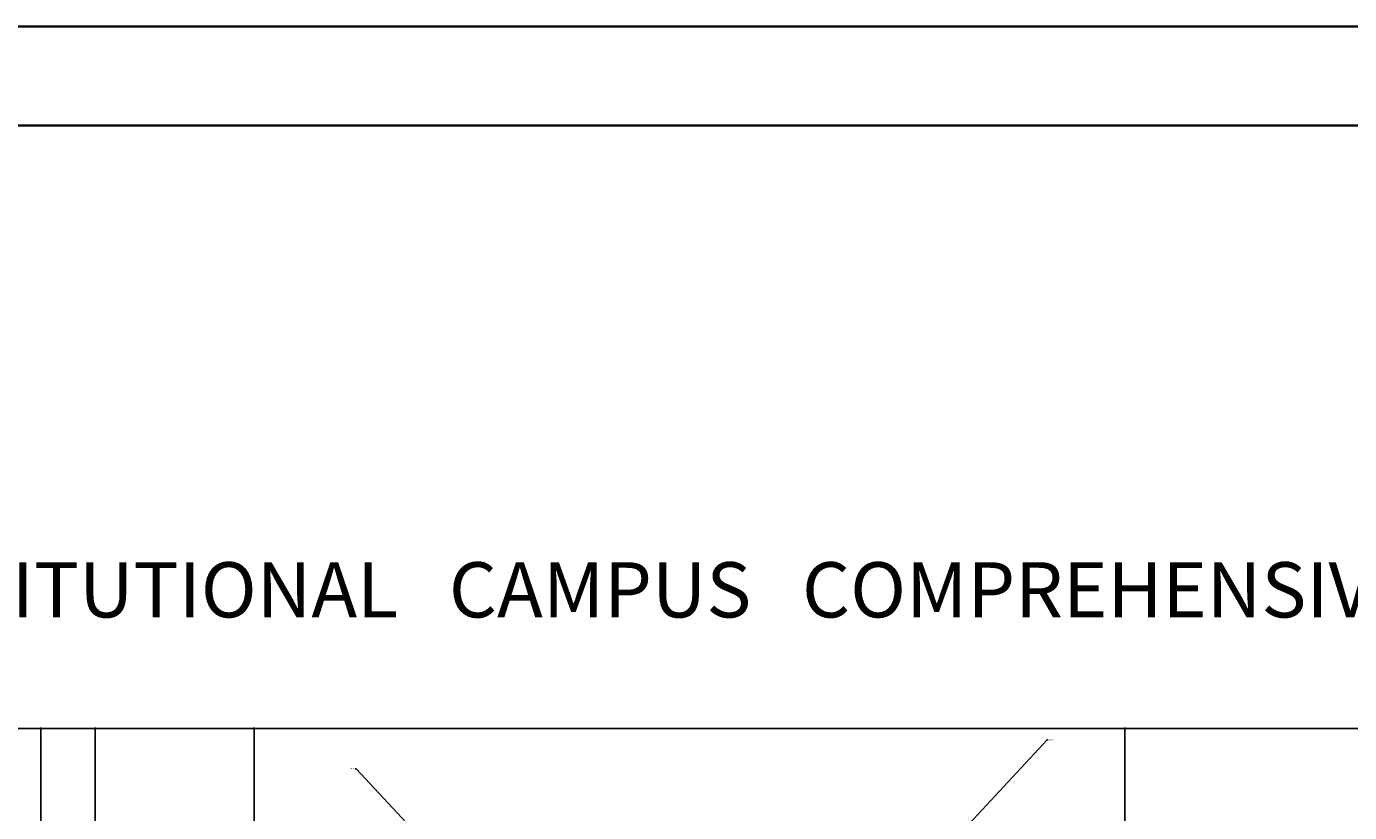
# Model space of a CAD drawing. Units: inches. Extents: x -279 to 364, y -385 to 335.
# Tile 8 of 9: x -60 to 168, y 199 to 335. Entities that reach past the tile are written whole.
import ezdxf

# ---------------------------------------------------------------- set-up
doc = ezdxf.new("R2010")
doc.units = ezdxf.units.IN
doc.header["$MEASUREMENT"] = 0
for name, color, linetype, lineweight in [('A-ANNO-DIMS', 2, 'Continuous', 18), ('A-ANNO-TEXT', 7, 'Continuous', 25), ('A-ANNO-TTLB', 7, 'Continuous', 35)]:
    doc.layers.add(name, color=color, linetype=linetype, lineweight=lineweight)
doc.styles.get("Standard").update_dxf_attribs({"font": 'arial.ttf'})
doc.dimstyles.get("Standard").update_dxf_attribs({"dimtxt": 0.18, "dimasz": 0.18, "dimexe": 0.18, "dimexo": 0.0625, "dimgap": 0.09, "dimtad": 0, "dimtih": 1, "dimtoh": 1, "dimdec": 4, "dimzin": 0, "dimdsep": 46, "dimtxsty": 'Standard', "dimcen": 0.09, "dimadec": 0, "dimazin": 0, "dimtfac": 1, "dimtdec": 4, "dimtofl": 0, "dimtmove": 0, "dimatfit": 3, "dimfxl": 1, "dimtolj": 1, "dimtzin": 0, "dimarcsym": 0})

# ---------------------------------------------------------------- blocks, each defined once
blk = doc.blocks.new('*D74')
at = {"layer": 'A-ANNO-DIMS', "color": 0, "lineweight": -2, "transparency": 16777216}
for p, q in [((-137.56, 76.08), (-137.56, 213.67)), ((-137.38, 213.49), (54.29, 213.49)), ((246.75, 213.49), (55.08, 213.49)), ((246.93, 76.27), (246.93, 213.67))]:
    blk.add_line(p, q, dxfattribs=at)
at = {"layer": 'A-ANNO-DIMS', "color": 0, "transparency": 16777216}
for points in [[(-137.38, 213.52), (-137.38, 213.46), (-137.56, 213.49)], [(246.75, 213.52), (246.75, 213.46), (246.93, 213.49)]]:
    blk.add_solid(points, dxfattribs=at)
at = {"layer": 'Defpoints', "color": 0, "transparency": 16777216}
for p in [(246.93, 213.49), (-137.56, 76.01), (246.93, 76.21)]:
    blk.add_point(p, dxfattribs=at)
at = {"layer": 'A-ANNO-DIMS', "color": 0, "transparency": 16777216, "insert": (54.68, 213.49), "char_height": 0.18, "attachment_point": 5}
blk.add_mtext('\\A1;384.5', dxfattribs=at)
blk = doc.blocks.new('*D89')
at = {"layer": 'A-ANNO-DIMS', "color": 0, "lineweight": -2, "transparency": 16777216}
for p, q in [((-57.96, 47.23), (-57.96, 213.67)), ((-57.78, 213.49), (-53.69, 213.49)), ((-48.8, 213.49), (-52.9, 213.49)), ((-48.62, 47.23), (-48.62, 213.67))]:
    blk.add_line(p, q, dxfattribs=at)
at = {"layer": 'A-ANNO-DIMS', "color": 0, "transparency": 16777216}
for points in [[(-57.78, 213.52), (-57.78, 213.46), (-57.96, 213.49)], [(-48.8, 213.52), (-48.8, 213.46), (-48.62, 213.49)]]:
    blk.add_solid(points, dxfattribs=at)
at = {"layer": 'Defpoints', "color": 0, "transparency": 16777216}
for p in [(-48.62, 213.49), (-57.96, 47.17), (-48.62, 47.17)]:
    blk.add_point(p, dxfattribs=at)
at = {"layer": 'A-ANNO-DIMS', "color": 0, "transparency": 16777216, "insert": (-53.29, 213.49), "char_height": 0.18, "attachment_point": 5}
blk.add_mtext('\\A1;9.335', dxfattribs=at)
blk = doc.blocks.new('*D93')
at = {"layer": 'A-ANNO-DIMS', "color": 0, "lineweight": -2, "transparency": 16777216}
for p, q in [((-21.19, 7.14), (-21.19, 213.67)), ((-21.01, 213.49), (53.45, 213.49)), ((128.81, 213.49), (54.36, 213.49)), ((128.99, 7.33), (128.99, 213.67))]:
    blk.add_line(p, q, dxfattribs=at)
at = {"layer": 'A-ANNO-DIMS', "color": 0, "transparency": 16777216}
for points in [[(-21.01, 213.52), (-21.01, 213.46), (-21.19, 213.49)], [(128.81, 213.52), (128.81, 213.46), (128.99, 213.49)]]:
    blk.add_solid(points, dxfattribs=at)
at = {"layer": 'Defpoints', "color": 0, "transparency": 16777216}
for p in [(128.99, 213.49), (-21.19, 7.08), (128.99, 7.27)]:
    blk.add_point(p, dxfattribs=at)
at = {"layer": 'A-ANNO-DIMS', "color": 0, "transparency": 16777216, "insert": (53.9, 213.49), "char_height": 0.18, "attachment_point": 5}
blk.add_mtext('\\A1;150.18', dxfattribs=at)
blk = doc.blocks.new('*D117')
at = {"layer": 'A-ANNO-DIMS', "color": 0, "lineweight": -2, "transparency": 16777216}
for p, q in [((115.61, 211.52), (74.41, 167.34)), ((115.79, 211.52), (115.61, 211.52)), ((5.33, 93.35), (5.51, 93.35)), ((5.42, 93.26), (5.42, 93.44))]:
    blk.add_line(p, q, dxfattribs=at)
at = {"layer": 'A-ANNO-DIMS', "color": 0, "transparency": 16777216}
blk.add_solid([(74.39, 167.36), (74.44, 167.32), (74.29, 167.21)], dxfattribs=at)
at = {"layer": 'Defpoints', "color": 0, "transparency": 16777216}
for p in [(74.29, 167.21), (5.42, 93.35)]:
    blk.add_point(p, dxfattribs=at)
at = {"layer": 'A-ANNO-DIMS', "color": 0, "transparency": 16777216, "insert": (116.34, 211.52), "char_height": 0.18, "attachment_point": 5}
blk.add_mtext('\\A1;R100.98', dxfattribs=at)
blk = doc.blocks.new('*D118')
at = {"layer": 'A-ANNO-DIMS', "color": 0, "lineweight": -2, "transparency": 16777216}
for p, q in [((-3.78, 206.52), (-3.6, 206.52)), ((-3.6, 206.52), (32.92, 167.57)), ((94.02, 102.29), (94.2, 102.29)), ((94.11, 102.2), (94.11, 102.38))]:
    blk.add_line(p, q, dxfattribs=at)
at = {"layer": 'A-ANNO-DIMS', "color": 0, "transparency": 16777216}
blk.add_solid([(32.94, 167.59), (32.9, 167.55), (33.04, 167.44)], dxfattribs=at)
at = {"layer": 'Defpoints', "color": 0, "transparency": 16777216}
for p in [(33.04, 167.44), (94.11, 102.29)]:
    blk.add_point(p, dxfattribs=at)
at = {"layer": 'A-ANNO-DIMS', "color": 0, "transparency": 16777216, "insert": (-4.26, 206.52), "char_height": 0.18, "attachment_point": 5}
blk.add_mtext('\\A1;R89.29', dxfattribs=at)

msp = doc.modelspace()

# ---------------------------------------------------------------- linework, layer by layer
at = {"layer": 'A-ANNO-TTLB'}
for points in [[(-279.2289, 334.6468), (364.0508, 334.6468), (364.0508, -385.2219), (-279.2289, -385.2219)], [(-267.2403, 317.5778), (348.1051, 317.5778), (348.1051, -370.8321), (-267.2403, -370.8321)]]:
    msp.add_lwpolyline(points, close=True, dxfattribs=at)

# ---------------------------------------------------------------- texts
at = {"layer": 'A-ANNO-TEXT'}
msp.add_text('MEGA   SCALE   INSTITUTIONAL   CAMPUS   COMPREHENSIVE   ELEVATION ', height=9.539438, dxfattribs=at).set_placement((-183.0703, 232.6637))

# ---------------------------------------------------------------- dimensions: what is measured, and where the dimension line sits
at = {"layer": 'A-ANNO-DIMS'}
for base, p1, p2, override, picture, middle in [((246.9255, 213.4896), (-137.5587, 76.0128), (246.9255, 76.2063), {"dimdec": 1, "dimlfac": 1, "dimrnd": 0, "dimzin": 0, "dimdsep": 46, "dimlunit": 2}, '*D74', (54.6834, 213.4896)), ((-48.6244, 213.4896), (-57.9596, 47.1683), (-48.6244, 47.1683), {"dimdec": 3, "dimlfac": 1, "dimrnd": 0, "dimzin": 0, "dimdsep": 46, "dimlunit": 2}, '*D89', (-53.292, 213.4896)), ((128.9927, 213.4896), (-21.1877, 7.0763), (128.9927, 7.2697), {"dimdec": 2, "dimlfac": 1, "dimrnd": 0, "dimzin": 0, "dimdsep": 46, "dimlunit": 2}, '*D93', (53.9025, 213.4896))]:
    dim = msp.add_linear_dim(base=base, p1=p1, p2=p2, dimstyle='Standard', override=override, dxfattribs=at)
    dim.commit()
    dim.dimension.update_dxf_attribs({"geometry": picture, "text_midpoint": middle})
for center, mpoint, picture, middle in [((5.4193, 93.3518), (74.291, 167.205), '*D117', (116.344, 211.517)), ((94.1065, 102.2938), (33.04, 167.436), '*D118', (-4.2599, 206.5213))]:
    dim = msp.add_radius_dim(center=center, mpoint=mpoint, dimstyle='Standard', override={"dimdec": 2, "dimlfac": 1, "dimrnd": 0, "dimzin": 0, "dimdsep": 46, "dimlunit": 2}, dxfattribs=at)
    dim.commit()
    dim.dimension.update_dxf_attribs({"geometry": picture, "text_midpoint": middle, "dimtype": 164})

doc.saveas('drawing.dxf')
